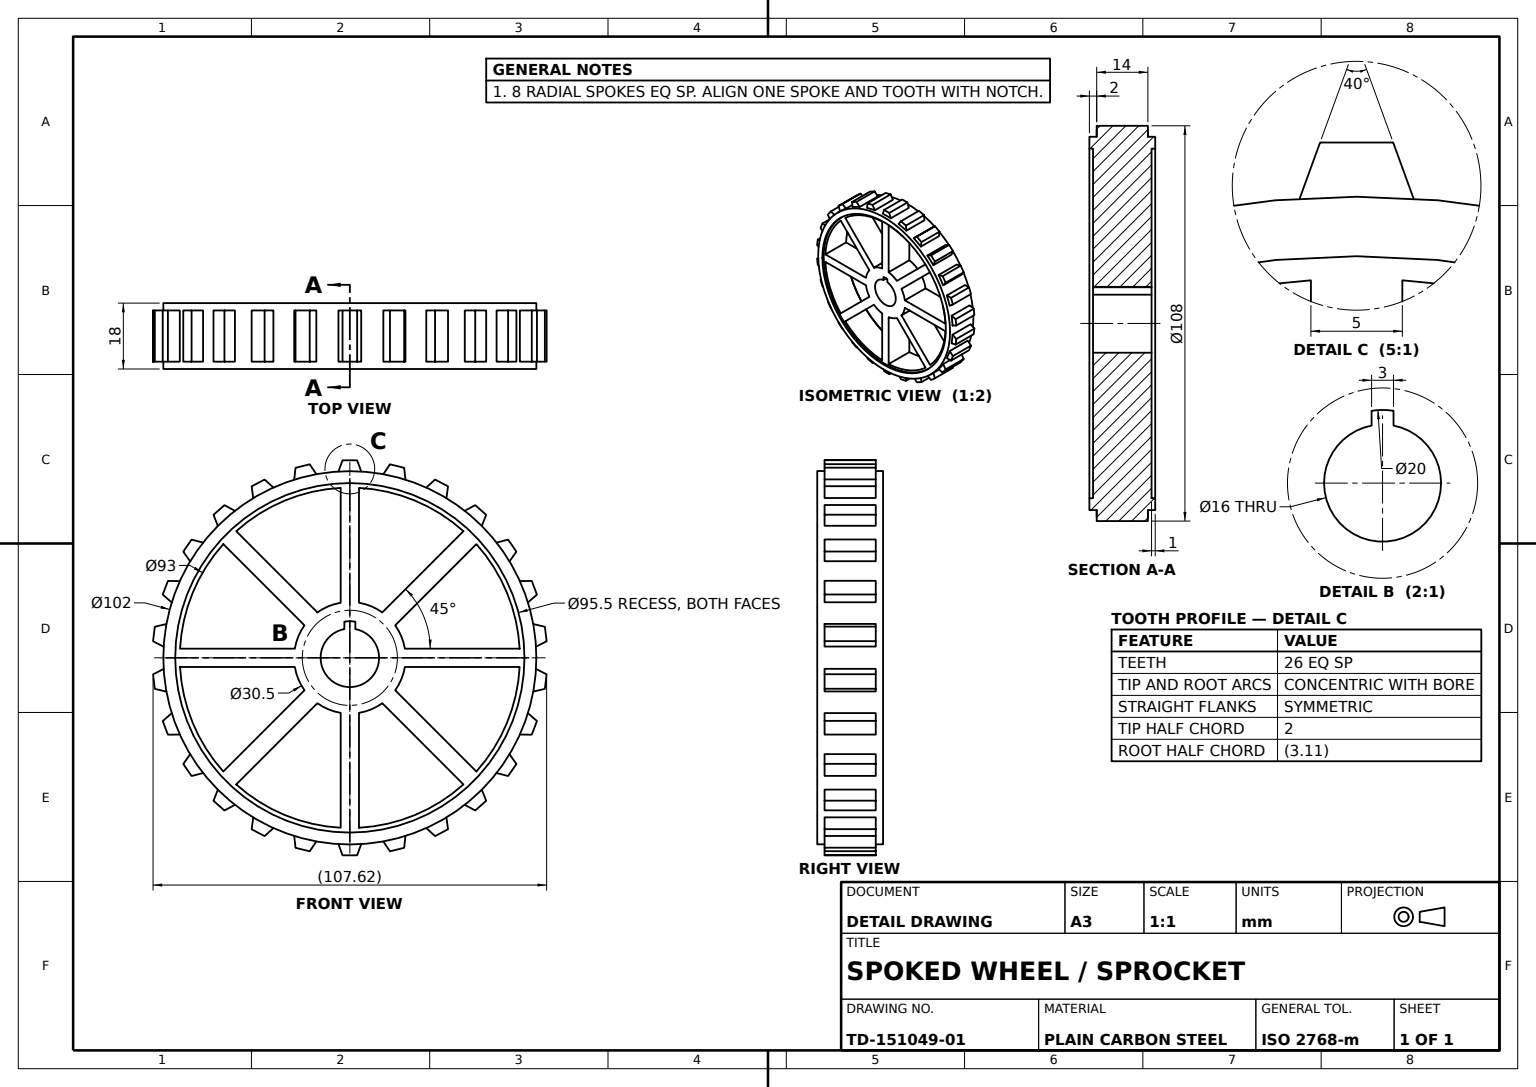
from build123d import *
from build123d.topology import SkipClean

# Parameters (mm, degrees)
HUB_SPOKES_RIM_SKETCH_R      = 51
HUB_SPOKES_RIM_SKETCH_R_2    = 8
WHEEL_BODY_8_SPOKES_DEPTH    = 9
TEETH_RING_26X_DEPTH         = 7
WEB_POCKETS_8X_DEPTH         = 78.894658104
HUB_CUT_20X16_DEPTH          = 79.329928898
FRONT_RECESS_SKETCH_95_5_R   = 47.75
FRONT_FACE_RECESS_95_5_DEPTH = 1
BACK_START                   = -1
BACK_RECESS_SKETCH_95_5_R    = 47.75
BACK_FACE_RECESS_95_5_DEPTH  = 1


with BuildPart() as part:
    # Hub Spokes Rim Sketch → Wheel Body 8 Spokes (new, symmetric)
    with BuildSketch(Plane.XY):
        Circle(HUB_SPOKES_RIM_SKETCH_R)
        Circle(HUB_SPOKES_RIM_SKETCH_R_2, mode=Mode.SUBTRACT)
        with BuildLine():
            Line((-2.5, 15.043686383), (-2.5, 46.432747065))
            ThreePointArc((-2.5, 46.432747065), (-17.794779605, 42.960398262), (-31.065143366, 34.600677272))
            Line((-31.065143366, 34.600677272), (-8.869725703, 12.405259609))
            ThreePointArc((-8.869725703, 12.405259609), (-5.835922344, 14.089162871), (-2.5, 15.043686383))
        make_face(mode=Mode.SUBTRACT)
        with BuildLine():
            Line((2.5, 46.432747065), (2.5, 15.043686383))
            ThreePointArc((2.5, 15.043686383), (5.835922344, 14.089162871), (8.869725703, 12.405259609))
            Line((8.869725703, 12.405259609), (31.065143366, 34.600677272))
            ThreePointArc((31.065143366, 34.600677272), (17.794779605, 42.960398262), (2.5, 46.432747065))
        make_face(mode=Mode.SUBTRACT)
        with BuildLine():
            Line((34.600677272, 31.065143366), (12.405259609, 8.869725703))
            ThreePointArc((12.405259609, 8.869725703), (14.089162871, 5.835922344), (15.043686383, 2.5))
            Line((15.043686383, 2.5), (46.432747065, 2.5))
            ThreePointArc((46.432747065, 2.5), (42.960398262, 17.794779605), (34.600677272, 31.065143366))
        make_face(mode=Mode.SUBTRACT)
        with BuildLine():
            Line((46.432747065, -2.5), (15.043686383, -2.5))
            ThreePointArc((15.043686383, -2.5), (14.089162871, -5.835922344), (12.405259609, -8.869725703))
            Line((12.405259609, -8.869725703), (34.600677272, -31.065143366))
            ThreePointArc((34.600677272, -31.065143366), (42.960398262, -17.794779605), (46.432747065, -2.5))
        make_face(mode=Mode.SUBTRACT)
        with BuildLine():
            Line((31.065143366, -34.600677272), (8.869725703, -12.405259609))
            ThreePointArc((8.869725703, -12.405259609), (5.835922344, -14.089162871), (2.5, -15.043686383))
            Line((2.5, -15.043686383), (2.5, -46.432747065))
            ThreePointArc((2.5, -46.432747065), (17.794779605, -42.960398262), (31.065143366, -34.600677272))
        make_face(mode=Mode.SUBTRACT)
        with BuildLine():
            Line((-2.5, -46.432747065), (-2.5, -15.043686383))
            ThreePointArc((-2.5, -15.043686383), (-5.835922344, -14.089162871), (-8.869725703, -12.405259609))
            Line((-8.869725703, -12.405259609), (-31.065143366, -34.600677272))
            ThreePointArc((-31.065143366, -34.600677272), (-17.794779605, -42.960398262), (-2.5, -46.432747065))
        make_face(mode=Mode.SUBTRACT)
        with BuildLine():
            Line((-34.600677272, -31.065143366), (-12.405259609, -8.869725703))
            ThreePointArc((-12.405259609, -8.869725703), (-14.089162871, -5.835922344), (-15.043686383, -2.5))
            Line((-15.043686383, -2.5), (-46.432747065, -2.5))
            ThreePointArc((-46.432747065, -2.5), (-42.960398262, -17.794779605), (-34.600677272, -31.065143366))
        make_face(mode=Mode.SUBTRACT)
        with BuildLine():
            Line((-46.432747065, 2.5), (-15.043686383, 2.5))
            ThreePointArc((-15.043686383, 2.5), (-14.089162871, 5.835922344), (-12.405259609, 8.869725703))
            Line((-12.405259609, 8.869725703), (-34.600677272, 31.065143366))
            ThreePointArc((-34.600677272, 31.065143366), (-42.960398262, 17.794779605), (-46.432747065, 2.5))
        make_face(mode=Mode.SUBTRACT)
    extrude(amount=WHEEL_BODY_8_SPOKES_DEPTH, both=True)

    # Teeth Profile Sketch 26x → Teeth Ring 26x (add, symmetric)
    with SkipClean():  # the faces are left unmerged after this step: merging them gives an invalid solid
        with BuildSketch(Plane.XY):
            with BuildLine():
                Line((10.972295652, 52.873516321), (9.159760804, 50.170696447))
                ThreePointArc((9.159760804, 50.170696447), (6.147370693, 50.628152579), (3.113038746, 50.904901432))
                Line((3.113038746, 50.904901432), (2, 53.962950253))
                ThreePointArc((2, 53.962950253), (0, 54), (-2, 53.962950253))
                Line((-2, 53.962950253), (-3.113038746, 50.904901432))
                ThreePointArc((-3.113038746, 50.904901432), (-6.147370693, 50.628152579), (-9.159760804, 50.170696447))
                Line((-9.159760804, 50.170696447), (-10.972295652, 52.873516321))
                ThreePointArc((-10.972295652, 52.873516321), (-12.923045872, 52.430858141), (-14.856062922, 51.916253664))
                Line((-14.856062922, 51.916253664), (-15.204919799, 48.680698577))
                ThreePointArc((-15.204919799, 48.680698577), (-18.084849239, 47.685828377), (-20.90022835, 46.520752949))
                Line((-20.90022835, 46.520752949), (-23.306921363, 48.711265808))
                ThreePointArc((-23.306921363, 48.711265808), (-25.09505129, 47.814625385), (-26.848745466, 46.852373119))
                Line((-26.848745466, 46.852373119), (-26.413146182, 43.627350467))
                ThreePointArc((-26.413146182, 43.627350467), (-28.971302083, 41.972177161), (-31.426050594, 40.167192385))
                Line((-31.426050594, 40.167192385), (-34.287033522, 41.718093584))
                ThreePointArc((-34.287033522, 41.718093584), (-35.808623545, 40.419580401), (-37.281076515, 39.065602951))
                Line((-37.281076515, 39.065602951), (-36.086336516, 36.038539328))
                ThreePointArc((-36.086336516, 36.038539328), (-38.174048157, 33.81925557), (-40.125505006, 31.479260601))
                Line((-40.125505006, 31.479260601), (-43.274507921, 32.3004174))
                ThreePointArc((-43.274507921, 32.3004174), (-44.441128758, 30.675496323), (-45.546766908, 29.008481937))
                Line((-45.546766908, 29.008481937), (-43.66232014, 26.355299277))
                ThreePointArc((-43.66232014, 26.355299277), (-45.158257308, 23.700881774), (-46.493010918, 20.961868614))
                Line((-46.493010918, 20.961868614), (-49.747025216, 21.005558364))
                ThreePointArc((-49.747025216, 21.005558364), (-50.490877105, 19.1486639), (-51.165444764, 17.265493394))
                Line((-51.165444764, 17.265493394), (-48.700808424, 15.140385031))
                ThreePointArc((-48.700808424, 15.140385031), (-49.518032689, 12.205098879), (-50.15851203, 9.226249016))
                Line((-50.15851203, 9.226249016), (-53.328426228, 8.489932628))
                ThreePointArc((-53.328426228, 8.489932628), (-53.606279201, 6.508980734), (-53.810572949, 4.519097132))
                Line((-53.810572949, 4.519097132), (-50.908982742, 3.045566639))
                ThreePointArc((-50.908982742, 3.045566639), (-51, 0), (-50.908982742, -3.045566639))
                Line((-50.908982742, -3.045566639), (-53.810572949, -4.519097132))
                ThreePointArc((-53.810572949, -4.519097132), (-53.606279201, -6.508980734), (-53.328426228, -8.489932628))
                Line((-53.328426228, -8.489932628), (-50.15851203, -9.226249016))
                ThreePointArc((-50.15851203, -9.226249016), (-49.518032689, -12.205098879), (-48.700808424, -15.140385031))
                Line((-48.700808424, -15.140385031), (-51.165444764, -17.265493394))
                ThreePointArc((-51.165444764, -17.265493394), (-50.490877105, -19.1486639), (-49.747025216, -21.005558364))
                Line((-49.747025216, -21.005558364), (-46.493010918, -20.961868614))
                ThreePointArc((-46.493010918, -20.961868614), (-45.158257308, -23.700881774), (-43.66232014, -26.355299277))
                Line((-43.66232014, -26.355299277), (-45.546766908, -29.008481937))
                ThreePointArc((-45.546766908, -29.008481937), (-44.441128758, -30.675496323), (-43.274507921, -32.3004174))
                Line((-43.274507921, -32.3004174), (-40.125505006, -31.479260601))
                ThreePointArc((-40.125505006, -31.479260601), (-38.174048157, -33.81925557), (-36.086336516, -36.038539328))
                Line((-36.086336516, -36.038539328), (-37.281076515, -39.065602951))
                ThreePointArc((-37.281076515, -39.065602951), (-35.808623545, -40.419580401), (-34.287033522, -41.718093584))
                Line((-34.287033522, -41.718093584), (-31.426050594, -40.167192385))
                ThreePointArc((-31.426050594, -40.167192385), (-28.971302083, -41.972177161), (-26.413146182, -43.627350467))
                Line((-26.413146182, -43.627350467), (-26.848745466, -46.852373119))
                ThreePointArc((-26.848745466, -46.852373119), (-25.09505129, -47.814625385), (-23.306921363, -48.711265808))
                Line((-23.306921363, -48.711265808), (-20.90022835, -46.520752949))
                ThreePointArc((-20.90022835, -46.520752949), (-18.084849239, -47.685828377), (-15.204919799, -48.680698577))
                Line((-15.204919799, -48.680698577), (-14.856062922, -51.916253664))
                ThreePointArc((-14.856062922, -51.916253664), (-12.923045872, -52.430858141), (-10.972295652, -52.873516321))
                Line((-10.972295652, -52.873516321), (-9.159760804, -50.170696447))
                ThreePointArc((-9.159760804, -50.170696447), (-6.147370693, -50.628152579), (-3.113038746, -50.904901432))
                Line((-3.113038746, -50.904901432), (-2, -53.962950253))
                ThreePointArc((-2, -53.962950253), (0, -54), (2, -53.962950253))
                Line((2, -53.962950253), (3.113038746, -50.904901432))
                ThreePointArc((3.113038746, -50.904901432), (6.147370693, -50.628152579), (9.159760804, -50.170696447))
                Line((9.159760804, -50.170696447), (10.972295652, -52.873516321))
                ThreePointArc((10.972295652, -52.873516321), (12.923045872, -52.430858141), (14.856062922, -51.916253664))
                Line((14.856062922, -51.916253664), (15.204919799, -48.680698577))
                ThreePointArc((15.204919799, -48.680698577), (18.084849239, -47.685828377), (20.90022835, -46.520752949))
                Line((20.90022835, -46.520752949), (23.306921363, -48.711265808))
                ThreePointArc((23.306921363, -48.711265808), (25.09505129, -47.814625385), (26.848745466, -46.852373119))
                Line((26.848745466, -46.852373119), (26.413146182, -43.627350467))
                ThreePointArc((26.413146182, -43.627350467), (28.971302083, -41.972177161), (31.426050594, -40.167192385))
                Line((31.426050594, -40.167192385), (34.287033522, -41.718093584))
                ThreePointArc((34.287033522, -41.718093584), (35.808623545, -40.419580401), (37.281076515, -39.065602951))
                Line((37.281076515, -39.065602951), (36.086336516, -36.038539328))
                ThreePointArc((36.086336516, -36.038539328), (38.174048157, -33.81925557), (40.125505006, -31.479260601))
                Line((40.125505006, -31.479260601), (43.274507921, -32.3004174))
                ThreePointArc((43.274507921, -32.3004174), (44.441128758, -30.675496323), (45.546766908, -29.008481937))
                Line((45.546766908, -29.008481937), (43.66232014, -26.355299277))
                ThreePointArc((43.66232014, -26.355299277), (45.158257308, -23.700881774), (46.493010918, -20.961868614))
                Line((46.493010918, -20.961868614), (49.747025216, -21.005558364))
                ThreePointArc((49.747025216, -21.005558364), (50.490877105, -19.1486639), (51.165444764, -17.265493394))
                Line((51.165444764, -17.265493394), (48.700808424, -15.140385031))
                ThreePointArc((48.700808424, -15.140385031), (49.518032689, -12.205098879), (50.15851203, -9.226249016))
                Line((50.15851203, -9.226249016), (53.328426228, -8.489932628))
                ThreePointArc((53.328426228, -8.489932628), (53.606279201, -6.508980734), (53.810572949, -4.519097132))
                Line((53.810572949, -4.519097132), (50.908982742, -3.045566639))
                ThreePointArc((50.908982742, -3.045566639), (51, 0), (50.908982742, 3.045566639))
                Line((50.908982742, 3.045566639), (53.810572949, 4.519097132))
                ThreePointArc((53.810572949, 4.519097132), (53.606279201, 6.508980734), (53.328426228, 8.489932628))
                Line((53.328426228, 8.489932628), (50.15851203, 9.226249016))
                ThreePointArc((50.15851203, 9.226249016), (49.518032689, 12.205098879), (48.700808424, 15.140385031))
                Line((48.700808424, 15.140385031), (51.165444764, 17.265493394))
                ThreePointArc((51.165444764, 17.265493394), (50.490877105, 19.1486639), (49.747025216, 21.005558364))
                Line((49.747025216, 21.005558364), (46.493010918, 20.961868614))
                ThreePointArc((46.493010918, 20.961868614), (45.158257308, 23.700881774), (43.66232014, 26.355299277))
                Line((43.66232014, 26.355299277), (45.546766908, 29.008481937))
                ThreePointArc((45.546766908, 29.008481937), (44.441128758, 30.675496323), (43.274507921, 32.3004174))
                Line((43.274507921, 32.3004174), (40.125505006, 31.479260601))
                ThreePointArc((40.125505006, 31.479260601), (38.174048157, 33.81925557), (36.086336516, 36.038539328))
                Line((36.086336516, 36.038539328), (37.281076515, 39.065602951))
                ThreePointArc((37.281076515, 39.065602951), (35.808623545, 40.419580401), (34.287033522, 41.718093584))
                Line((34.287033522, 41.718093584), (31.426050594, 40.167192385))
                ThreePointArc((31.426050594, 40.167192385), (28.971302083, 41.972177161), (26.413146182, 43.627350467))
                Line((26.413146182, 43.627350467), (26.848745466, 46.852373119))
                ThreePointArc((26.848745466, 46.852373119), (25.09505129, 47.814625385), (23.306921363, 48.711265808))
                Line((23.306921363, 48.711265808), (20.90022835, 46.520752949))
                ThreePointArc((20.90022835, 46.520752949), (18.084849239, 47.685828377), (15.204919799, 48.680698577))
                Line((15.204919799, 48.680698577), (14.856062922, 51.916253664))
                ThreePointArc((14.856062922, 51.916253664), (12.923045872, 52.430858141), (10.972295652, 52.873516321))
            make_face()
        extrude(amount=TEETH_RING_26X_DEPTH, both=True)

    # Web Pockets Sketch 8x → Web Pockets 8x (cut, through all)
    with SkipClean():  # the faces are left unmerged after this step: merging them gives an invalid solid
        with BuildSketch(Plane.XY.offset(7)):
            with BuildLine():
                Line((2.5, 15.043686383), (2.5, 46.432747065))
                ThreePointArc((2.5, 46.432747065), (17.794779605, 42.960398262), (31.065143366, 34.600677272))
                Line((31.065143366, 34.600677272), (8.869725703, 12.405259609))
                ThreePointArc((8.869725703, 12.405259609), (5.835922344, 14.089162871), (2.5, 15.043686383))
            make_face()
            with BuildLine():
                Line((12.405259609, 8.869725703), (34.600677272, 31.065143366))
                ThreePointArc((34.600677272, 31.065143366), (42.960398262, 17.794779605), (46.432747065, 2.5))
                Line((46.432747065, 2.5), (15.043686383, 2.5))
                ThreePointArc((15.043686383, 2.5), (14.089162871, 5.835922344), (12.405259609, 8.869725703))
            make_face()
            with BuildLine():
                Line((15.043686383, -2.5), (46.432747065, -2.5))
                ThreePointArc((46.432747065, -2.5), (42.960398262, -17.794779605), (34.600677272, -31.065143366))
                Line((34.600677272, -31.065143366), (12.405259609, -8.869725703))
                ThreePointArc((12.405259609, -8.869725703), (14.089162871, -5.835922344), (15.043686383, -2.5))
            make_face()
            with BuildLine():
                Line((8.869725703, -12.405259609), (31.065143366, -34.600677272))
                ThreePointArc((31.065143366, -34.600677272), (17.794779605, -42.960398262), (2.5, -46.432747065))
                Line((2.5, -46.432747065), (2.5, -15.043686383))
                ThreePointArc((2.5, -15.043686383), (5.835922344, -14.089162871), (8.869725703, -12.405259609))
            make_face()
            with BuildLine():
                Line((-2.5, -15.043686383), (-2.5, -46.432747065))
                ThreePointArc((-2.5, -46.432747065), (-17.794779605, -42.960398262), (-31.065143366, -34.600677272))
                Line((-31.065143366, -34.600677272), (-8.869725703, -12.405259609))
                ThreePointArc((-8.869725703, -12.405259609), (-5.835922344, -14.089162871), (-2.5, -15.043686383))
            make_face()
            with BuildLine():
                Line((-12.405259609, -8.869725703), (-34.600677272, -31.065143366))
                ThreePointArc((-34.600677272, -31.065143366), (-42.960398262, -17.794779605), (-46.432747065, -2.5))
                Line((-46.432747065, -2.5), (-15.043686383, -2.5))
                ThreePointArc((-15.043686383, -2.5), (-14.089162871, -5.835922344), (-12.405259609, -8.869725703))
            make_face()
            with BuildLine():
                Line((-15.043686383, 2.5), (-46.432747065, 2.5))
                ThreePointArc((-46.432747065, 2.5), (-42.960398262, 17.794779605), (-34.600677272, 31.065143366))
                Line((-34.600677272, 31.065143366), (-12.405259609, 8.869725703))
                ThreePointArc((-12.405259609, 8.869725703), (-14.089162871, 5.835922344), (-15.043686383, 2.5))
            make_face()
            with BuildLine():
                Line((-8.869725703, 12.405259609), (-31.065143366, 34.600677272))
                ThreePointArc((-31.065143366, 34.600677272), (-17.794779605, 42.960398262), (-2.5, 46.432747065))
                Line((-2.5, 46.432747065), (-2.5, 15.043686383))
                ThreePointArc((-2.5, 15.043686383), (-5.835922344, 14.089162871), (-8.869725703, 12.405259609))
            make_face()
        extrude(amount=-WEB_POCKETS_8X_DEPTH, mode=Mode.SUBTRACT)

    # Hub Cut Sketch 20x16 → Hub Cut 20x16 (cut, through all)
    with SkipClean():  # the faces are left unmerged after this step: merging them gives an invalid solid
        with BuildSketch(Plane.XY.offset(9)):
            with BuildLine():
                Line((1.5, 9.886859967), (1.5, 7.858116823))
                ThreePointArc((1.5, 7.858116823), (0, -8), (-1.5, 7.858116823))
                Line((-1.5, 7.858116823), (-1.5, 9.886859967))
                ThreePointArc((-1.5, 9.886859967), (0, 10), (1.5, 9.886859967))
            make_face()
        extrude(amount=-HUB_CUT_20X16_DEPTH, mode=Mode.SUBTRACT)

    # Front Recess Sketch Ø95.5 → Front Face Recess Ø95.5 (cut)
    with SkipClean():  # the faces are left unmerged after this step: merging them gives an invalid solid
        with BuildSketch(Plane.XY.offset(9)):
            Circle(FRONT_RECESS_SKETCH_95_5_R)
        extrude(amount=-FRONT_FACE_RECESS_95_5_DEPTH, mode=Mode.SUBTRACT)

    # Back Recess Sketch Ø95.5 → Back Face Recess Ø95.5 (cut)
    with SkipClean():  # the faces are left unmerged after this step: merging them gives an invalid solid
        with BuildSketch(Plane(origin=(0, 0, -9), x_dir=(-1, 0, 0), z_dir=(0, 0, -1)).offset(BACK_START)):
            with Locations(Location((0, 0, 0), (0, 0, 180))):
                Circle(BACK_RECESS_SKETCH_95_5_R)
        extrude(amount=BACK_FACE_RECESS_95_5_DEPTH, mode=Mode.SUBTRACT)


solid = part.part
